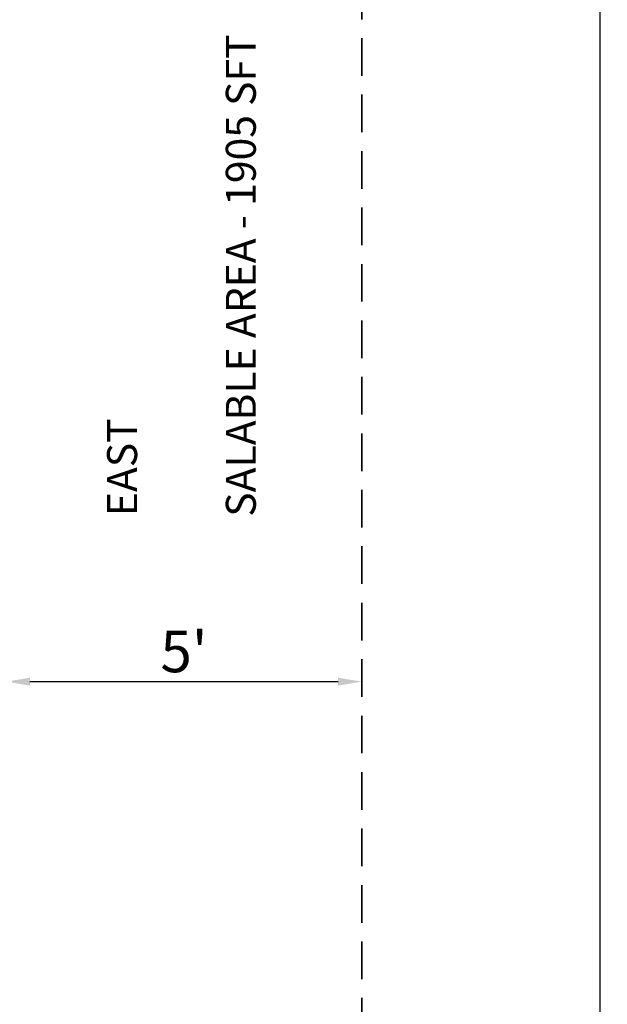
# Model space of a CAD drawing. Units: inches. Extents: x -7 to 1228, y -146 to 1091.
# Tile 40 of 88: x 1129 to 1228, y 34 to 200. Entities that reach past the tile are written whole.
import ezdxf

# ---------------------------------------------------------------- set-up
doc = ezdxf.new("R2010")
doc.units = ezdxf.units.IN
doc.linetypes.add('DASHED2', pattern=[9.525, 6.35, -3.175])
for name, color, linetype, lineweight in [('A-ANNO-DIMS', 2, 'Continuous', 18), ('A-ANNO-TEXT', 7, 'Continuous', 18), ('C-PROP', 1, 'DASHED2', 35)]:
    doc.layers.add(name, color=color, linetype=linetype, lineweight=lineweight)
doc.styles.get("Standard").update_dxf_attribs({"font": 'arial.ttf'})
doc.dimstyles.new('ISO-25', dxfattribs={"dimtxt": 7, "dimasz": 4, "dimexe": 1.25, "dimexo": 0.625, "dimtad": 1, "dimdec": 1, "dimlunit": 3, "dimtxsty": 'Standard', "dimcen": 2.5, "dimadec": 0, "dimazin": 0, "dimtfac": 1, "dimtdec": 1, "dimtmove": 1, "dimatfit": 3, "dimfxl": 1, "dimarcsym": 0})

# ---------------------------------------------------------------- blocks, each defined once
blk = doc.blocks.new('*D12')
at = {"layer": 'A-ANNO-DIMS', "color": 0, "lineweight": -2, "transparency": 16777216}
for p, q in [((1187.62, 1061), (1228.45, 1061)), ((1227.2, 1057), (1227.2, 4)), ((1187.62, 0), (1228.45, 0))]:
    blk.add_line(p, q, dxfattribs=at)
at = {"layer": 'A-ANNO-DIMS', "color": 0, "transparency": 16777216}
for points in [[(1226.53, 1057), (1227.86, 1057), (1227.2, 1061)], [(1226.53, 4), (1227.86, 4), (1227.2, 0)]]:
    blk.add_solid(points, dxfattribs=at)
at = {"layer": 'Defpoints', "color": 0, "transparency": 16777216}
for p in [(1187, 1061), (1187, 0), (1227.2, 0)]:
    blk.add_point(p, dxfattribs=at)
at = {"layer": 'A-ANNO-DIMS', "color": 0, "transparency": 16777216, "insert": (1223, 530.5), "char_height": 7, "attachment_point": 5, "rotation": 90}
blk.add_mtext('88\'-5"', dxfattribs=at)
blk = doc.blocks.new('*D16')
at = {"layer": 'A-ANNO-DIMS', "color": 0, "lineweight": -2, "transparency": 16777216}
for p, q in [((1127, 88.08), (1127, 87.04)), ((1131, 88.29), (1183, 88.29)), ((1187, 88.08), (1187, 87.04))]:
    blk.add_line(p, q, dxfattribs=at)
at = {"layer": 'A-ANNO-DIMS', "color": 0, "transparency": 16777216}
for points in [[(1131, 88.96), (1131, 87.62), (1127, 88.29)], [(1183, 88.96), (1183, 87.62), (1187, 88.29)]]:
    blk.add_solid(points, dxfattribs=at)
at = {"layer": 'Defpoints', "color": 0, "transparency": 16777216}
for p in [(1127, 88.71), (1187, 88.71), (1187, 88.29)]:
    blk.add_point(p, dxfattribs=at)
at = {"layer": 'A-ANNO-DIMS', "color": 0, "transparency": 16777216, "insert": (1157, 92.47), "char_height": 7, "attachment_point": 5}
blk.add_mtext("5'", dxfattribs=at)

msp = doc.modelspace()

# ---------------------------------------------------------------- linework, layer by layer
at = {"layer": 'C-PROP'}
msp.add_line((1187, 0), (1187, 1061), dxfattribs=at)

# ---------------------------------------------------------------- texts
at = {"layer": 'A-ANNO-TEXT', "attachment_point": 1, "rotation": 90}
for s, insert, char_height in [('{SALABLE AREA - 1905 SFT}', (1164.06, 116.11), 5.0568), ('EAST', (1144.02, 116.21), 5.057)]:
    msp.add_mtext_dynamic_manual_height_columns(s, width=137.2821, gutter_width=25.28, heights=[0], dxfattribs=dict(at, insert=insert, char_height=char_height))

# ---------------------------------------------------------------- dimensions: what is measured, and where the dimension line sits
at = {"layer": 'A-ANNO-DIMS'}
dim = msp.add_linear_dim(base=(1227.2, 0), p1=(1187, 1061), p2=(1187, 0), angle=90, dimstyle='ISO-25', override={"dimclrd": 0, "dimclre": 0, "dimclrt": 0}, dxfattribs=at)
dim.commit()
dim.dimension.update_dxf_attribs({"geometry": '*D12', "text_midpoint": (1223, 530.5)})
dim = msp.add_linear_dim(base=(1187, 88.29), p1=(1127, 88.71), p2=(1187, 88.71), dimstyle='ISO-25', override={"dimclrd": 0, "dimclre": 0, "dimclrt": 0}, dxfattribs=at)
dim.commit()
dim.dimension.update_dxf_attribs({"geometry": '*D16', "text_midpoint": (1157, 92.47)})

doc.saveas('drawing.dxf')
